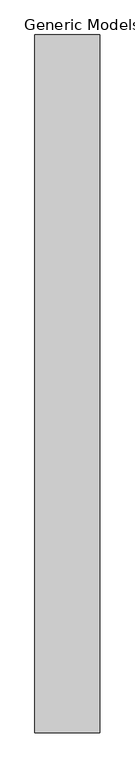
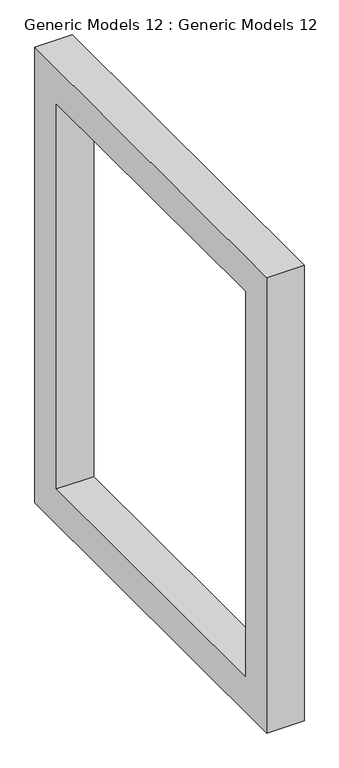
"""IFC4 building model written with IfcOpenShell, lengths in millimetres: proxy geometry, Generic Models 12 : Generic Models 12."""

from ifc_helpers import new_model, si_unit, frame, origin, place, context, project, spatial, polyline, outline, extrude, source, transform, mapped, element, save


def generic_models_12_generic_models_12_6289c3a4(model_context):
    return source(origin(), model_context, "Body", "SweptSolid", [
        extrude(outline(polyline([(1408.2655883, 2952.75), (1408.2655883, 987.4676291), (-230.0344117, 987.4676291), (-230.0344117, 2952.75), (1408.2655883, 2952.75)]), holes=[polyline([(1255.8655883, 2800.35), (-77.6344117, 2800.35), (-77.6344117, 1139.8676291), (1255.8655883, 1139.8676291), (1255.8655883, 2800.35)])]), frame((66.1413992, 0.0, 0.0), z_axis=(1.0, 0.0, 0.0), x_axis=(0.0, 1.0, 0.0)), (0.0, 0.0, 1.0), 152.4),
    ])


if __name__ == "__main__":
    model = new_model("IFC4")
    model_context = context("Model", 3, world=origin())
    ifc_project = project(units=[si_unit("LENGTHUNIT", "METRE", prefix="MILLI")], contexts=[model_context])
    site = spatial("IfcSite", under=ifc_project)
    building = spatial("IfcBuilding", under=site)
    placement = place(None, origin())
    generic_models_12_generic_models_12_shape = generic_models_12_generic_models_12_6289c3a4(model_context)
    element("IfcBuildingElementProxy", 1, Name="Generic Models 12 : Generic Models 12", ObjectType="Generic Models 12 : Generic Models 12", at=placement, inside=building, context=model_context, shape_type="MappedRepresentation", body=[
        mapped(generic_models_12_generic_models_12_shape, transform((0.0, 0.0, 0.0), x_axis=(1.0, 0.0, 0.0), y_axis=(0.0, 1.0, 0.0), z_axis=(0.0, 0.0, 1.0))),
    ])
    save(model, "model.ifc")

# Revit data of these elements
# Element 1 (IfcBuildingElementProxy, "Generic Models 12 : Generic Models 12")
#   Materials on its faces: "feature frame"
# Materials
#   "feature frame": class "Generic", colour RGB 120 120 120, transparency 0, Cost = 0
